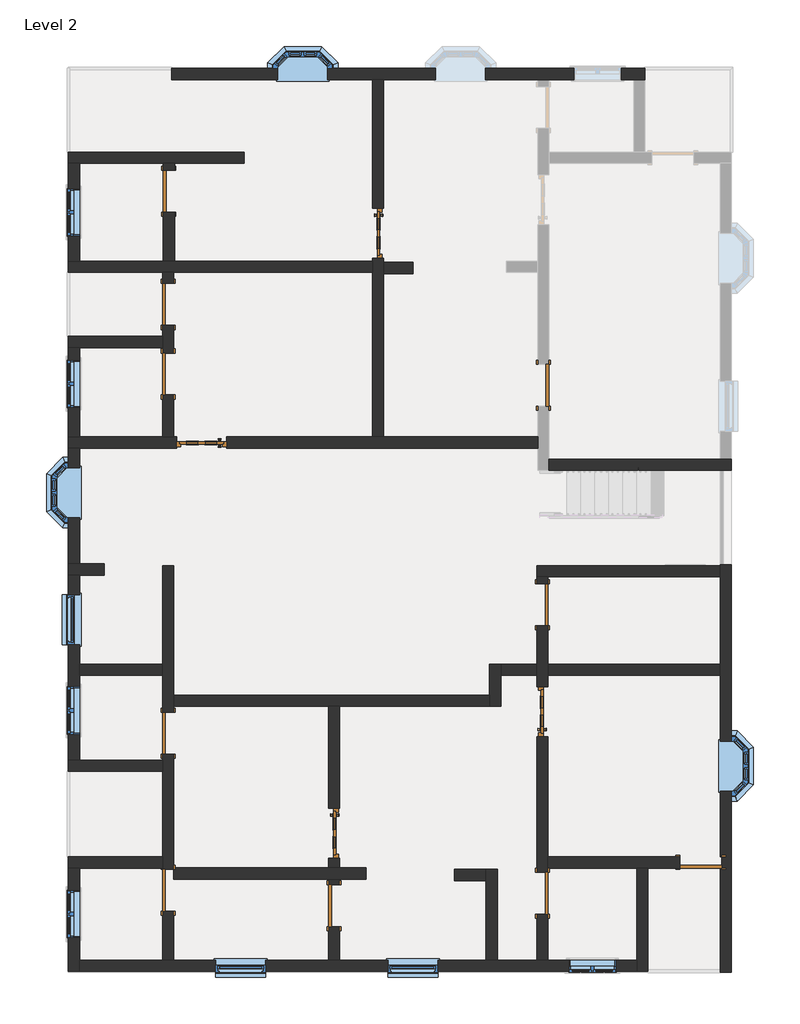
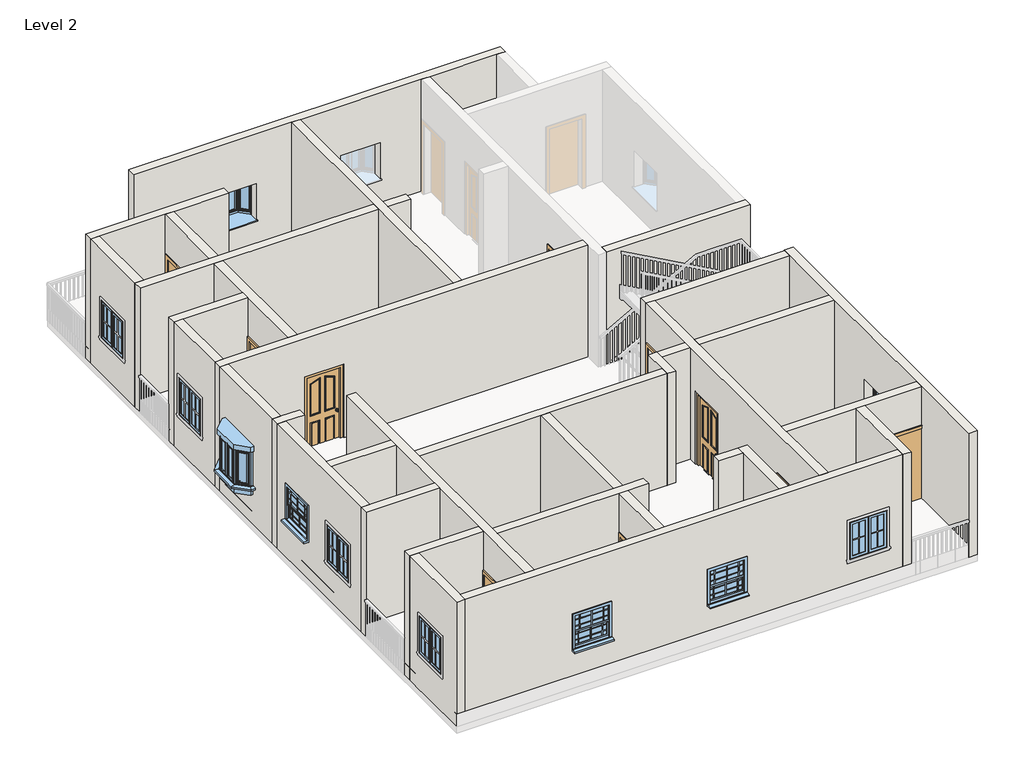
# One storey, part 1 of 4: 34 walls, 14 doors, 11 windows.
# Revit data of these elements (continued)
# Elements 15, 17, 18 (IfcWall, "Generic - 4.5\"") (continued)
#   Top Constraint = Level 3
#   Materials on its faces: "Default Wall", "Brick, Soldier Course"
# Elements 16, 20, 27, 31 (IfcWall, "Generic - 4.5\"")
#   Top Offset = 0' - 0"
#   Base Offset = 0' - 0"
#   wall height = 10' - 0"
#   Phase Created = New Construction
#   Base Constraint = Level 2
#   Top Constraint = Level 3
#   Materials on its faces: "Default Wall", "Parking Stripe"
# Elements 19, 21, 22, 30 (IfcWall, "Generic - 4.5\"")
#   Top Offset = 0' - 0"
#   Base Offset = 0' - 0"
#   wall height = 10' - 0"
#   Phase Created = New Construction
#   Base Constraint = Level 2
#   Top Constraint = Level 3
#   Materials on its faces: "Default Wall", "Earth"
# Element 23 (IfcWall, "Generic - 4.5\"")
#   Top Offset = 0' - 0"
#   Base Offset = 0' - 0"
#   wall height = 10' - 0"
#   Phase Created = New Construction
#   Base Constraint = Level 2
#   Top Constraint = Level 3
#   Materials on its faces: "Default Wall", "Earth", "Door - Frame/Mullion"
# Elements 24, 25, 26, 29, 32, 33, 34, 35, 36, 37, 38, 39, 40 (IfcWall, "Generic - 4.5\"")
#   Top Offset = 0' - 0"
#   Base Offset = 0' - 0"
#   wall height = 10' - 0"
#   Phase Created = New Construction
#   Base Constraint = Level 2
#   Top Constraint = Level 3
#   Materials on its faces: "Default Wall"
# Element 28 (IfcWall, "Generic - 4.5\"")
#   Top Offset = 0' - 0"
#   Base Offset = 0' - 0"
#   wall height = 10' - 0"
#   Phase Created = New Construction
#   Base Constraint = Level 2
#   Top Constraint = Level 3
#   Materials on its faces: "Default Wall", "Parking Stripe", "Cherry"
# Element 41 (IfcWall, "Generic - 9\"")
#   Top Offset = 0' - 0"
#   Base Offset = 0' - 0"
#   wall height = 10' - 0"
#   Phase Created = New Construction
#   Base Constraint = Level 2
#   Top Constraint = Level 3
#   Materials on its faces: "Default Wall", "Door - Panel", "Cherry", "Parking Stripe"
# Element 42 (IfcWall, "Generic - 9\"")
#   Top Offset = 0' - 0"
#   Base Offset = 0' - 0"
#   wall height = 10' - 0"
#   Phase Created = New Construction
#   Base Constraint = Level 2
#   Top Constraint = Level 3
#   Materials on its faces: "Default Wall", "Door - Frame/Mullion", "Parking Stripe"
# Element 43 (IfcWall, "Generic - 9\"")
#   Top Offset = 0' - 0"
#   Base Offset = 0' - 0"
#   wall height = 10' - 0"
#   Phase Created = New Construction
#   Base Constraint = Level 2
#   Top Constraint = Level 3
#   Materials on its faces: "Default Wall", "Parking Stripe"
# Elements 44, 45, 48 (IfcWall, "Generic - 9\"")
#   Top Offset = 0' - 0"
#   Base Offset = 0' - 0"
#   wall height = 10' - 0"
#   Phase Created = New Construction
#   Base Constraint = Level 2
#   Top Constraint = Level 3
#   Materials on its faces: "Default Wall", "Earth"
# Element 46 (IfcWall, "Generic - 9\"")
#   Top Offset = 0' - 0"
#   Base Offset = 0' - 0"
#   wall height = 10' - 0"
#   Phase Created = New Construction
#   Base Constraint = Level 2
#   Top Constraint = Level 3
#   Materials on its faces: "Default Wall", "Parking Stripe", "Cherry"
# Element 47 (IfcWall, "Generic - 9\"")
#   Top Offset = 0' - 0"
#   Base Offset = 0' - 0"
#   wall height = 10' - 0"
#   Phase Created = New Construction
#   Base Constraint = Level 2
#   Top Constraint = Level 3
#   Materials on its faces: "Default Wall", "Cherry"
# Element 49 (IfcWindow, "910x910mm")
#   Mark = "16"
#   Phase Created = New Construction
#   Materials on its faces: "Window Frame", "Glass"
# Element 50 (IfcWindow, "910x910mm")
#   Mark = "19"
#   Phase Created = New Construction
#   Materials on its faces: "Window Frame", "Glass"
# Element 51 (IfcWindow, "910x910mm")
#   Mark = "20"
#   Phase Created = New Construction
#   Materials on its faces: "Window Frame", "Glass"
# Element 52 (IfcWindow, "Window-Casement-Double : 34\" x 36\"")
#   Mark = "25"
#   Window Inset = 0' - 0"
#   Interior Wall Closure = 0' - 2 1/4"
#   Frame Extension = 0' - 0 1/4"
#   Exterior Wall Closure = 0' - 1 1/4"
#   Interior Trim Visibility = yes
#   Exterior Trim Visibility = yes
#   Phase Created = New Construction
#   Materials on its faces: "Wood - Stained", "Glass", "Clad - White"
# Element 53 (IfcWindow, "Window-Casement-Double : 34\" x 36\"")
#   Mark = "26"
#   Window Inset = 0' - 0"
#   Interior Wall Closure = 0' - 2 1/4"
#   Frame Extension = 0' - 0 1/4"
#   Exterior Wall Closure = 0' - 1 1/4"
#   Interior Trim Visibility = yes
#   Exterior Trim Visibility = yes
#   Phase Created = New Construction
#   Materials on its faces: "Wood - Stained", "Glass", "Clad - White"
# Element 54 (IfcWindow, "Window-Casement-Double : 34\" x 36\"")
#   Mark = "28"
#   Window Inset = 0' - 0"
#   Interior Wall Closure = 0' - 2 1/4"
#   Frame Extension = 0' - 0 1/4"
#   Exterior Wall Closure = 0' - 1 1/4"
#   Interior Trim Visibility = yes
#   Exterior Trim Visibility = yes
#   Phase Created = New Construction
#   Materials on its faces: "Wood - Stained", "Glass", "Clad - White"
# Element 55 (IfcWindow, "Window-Casement-Double : 34\" x 36\"")
#   Mark = "29"
#   Window Inset = 0' - 0"
#   Interior Wall Closure = 0' - 2 1/4"
#   Frame Extension = 0' - 0 1/4"
#   Exterior Wall Closure = 0' - 1 1/4"
#   Interior Trim Visibility = yes
#   Exterior Trim Visibility = yes
#   Phase Created = New Construction
#   Materials on its faces: "Wood - Stained", "Glass", "Clad - White"
# Element 56 (IfcWindow, "Window-Casement-Double : 34\" x 36\"")
#   Mark = "30"
#   Window Inset = 0' - 0"
#   Interior Wall Closure = 0' - 2 1/4"
#   Frame Extension = 0' - 0 1/4"
#   Exterior Wall Closure = 0' - 1 1/4"
#   Interior Trim Visibility = yes
#   Exterior Trim Visibility = yes
#   Phase Created = New Construction
#   Materials on its faces: "Wood - Stained", "Glass", "Clad - White"
# Element 57 (IfcWindow, "Windows_Sash_w-Bars_1 : 910x910mm")
#   Mark = "21"
#   Phase Created = New Construction
#   Materials on its faces: "Window Frame", "Glass"
# Element 58 (IfcWindow, "Windows_Sash_w-Bars_1 : 910x910mm")
#   Mark = "22"
#   Phase Created = New Construction
#   Materials on its faces: "Window Frame", "Glass"
# Element 59 (IfcWindow, "Windows_Sash_w-Bars_1 : 910x910mm")
#   Mark = "23"
#   Phase Created = New Construction
#   Materials on its faces: "Window Frame", "Glass"
# Materials
#   "Door - Glazing": colour RGB 0 0 255, transparency 0.75
#   "Door - Panel": class "Wood", colour RGB 210 159 95, transparency 0, Cost = 0
#   "Door - Frame/Mullion": class "Wood", colour RGB 212 179 113, transparency 0
#   "Door - Handle": colour RGB 247 247 247, transparency 0
#   "Door - Frame": colour RGB 118 70 51, transparency 0, Cost = 0
#   "Window Frame": colour RGB 249 249 249, transparency 0
#   "Glass": class "Glass", colour RGB 0 128 192, transparency 0.75, Description = "Soda Lime Glass", Cost = 0
#   "Wood - Stained": class "Wood", colour RGB 224 178 126, transparency 0, Cost = 0
#   "Clad - White": class "Wood", colour RGB 242 242 238, transparency 0, Cost = 0
#   "Default Wall": colour RGB 128 128 128, transparency 0, Cost = 0
#   "Brick, Soldier Course": class "Masonry", colour RGB 170 98 104, transparency 0, Description = "Common brick soldier coursed", Cost = 0
#   "Parking Stripe": class "Paint", colour RGB 250 250 91, transparency 0, Cost = 0
#   "Earth": class "Generic", colour RGB 97 75 62, transparency 0, Description = "Soil", Cost = 0
#   "Cherry": class "Wood", colour RGB 226 177 128, transparency 0, Description = "Prunus Serotina", Cost = 0
